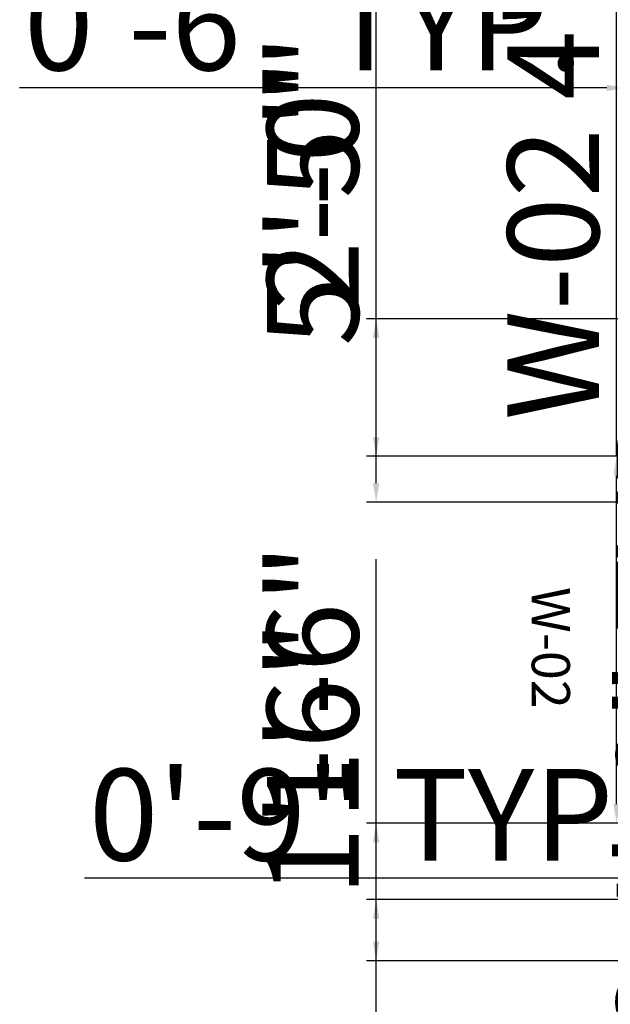
# Model space of a CAD drawing. Units: inches. Extents: x 2386 to 3029, y 792 to 1465.
# Tile 6 of 12: x 2386 to 2463, y 1140 to 1269. Entities that reach past the tile are written whole.
import ezdxf

# ---------------------------------------------------------------- set-up
doc = ezdxf.new("R2010")
doc.units = ezdxf.units.IN
doc.layers.add('A-DIMS', color=1, linetype='Continuous', lineweight=18)
doc.layers.add('A-TEXT', color=4, linetype='Continuous', lineweight=25)
doc.styles.get("Standard").update_dxf_attribs({"font": 'arial.ttf'})
doc.dimstyles.new('ISO-25', dxfattribs={"dimtxt": 12, "dimasz": 2.5, "dimexe": 1.25, "dimexo": 0.625, "dimtad": 1, "dimlunit": 4, "dimtxsty": 'Standard', "dimcen": 2.5, "dimadec": 0, "dimazin": 0, "dimtfac": 1, "dimtmove": 0, "dimatfit": 3, "dimfxl": 1, "dimarcsym": 0})

# ---------------------------------------------------------------- blocks, each defined once
blk = doc.blocks.new('*D38')
at = {"layer": 'A-DIMS', "color": 0, "lineweight": -2, "transparency": 16777216}
for p, q in [((2471.82, 1342.95), (2483.24, 1342.95)), ((2481.99, 1340.45), (2481.99, 1273.45)), ((2471.82, 1270.95), (2483.24, 1270.95)), ((2481.99, 1270.95), (2481.99, 1095.04))]:
    blk.add_line(p, q, dxfattribs=at)
at = {"layer": 'A-DIMS', "color": 0, "transparency": 16777216}
for points in [[(2481.57, 1340.45), (2482.41, 1340.45), (2481.99, 1342.95)], [(2481.57, 1273.45), (2482.41, 1273.45), (2481.99, 1270.95)]]:
    blk.add_solid(points, dxfattribs=at)
at = {"layer": 'Defpoints', "color": 0, "transparency": 16777216}
for p in [(2471.19, 1342.95), (2471.19, 1270.95), (2481.99, 1270.95)]:
    blk.add_point(p, dxfattribs=at)
at = {"layer": 'A-DIMS', "color": 0, "transparency": 16777216, "insert": (2475.16, 1181.74), "char_height": 12, "attachment_point": 5, "rotation": 90}
blk.add_mtext('HOOD W-01 6\'-0" TYP.', dxfattribs=at)
blk = doc.blocks.new('*D39')
at = {"layer": 'A-DIMS', "color": 0, "lineweight": -2, "transparency": 16777216}
for p, q in [((2465.19, 1270.32), (2465.19, 1258.9)), ((2471.19, 1270.32), (2471.19, 1258.9)), ((2462.69, 1260.15), (2385.79, 1260.15)), ((2471.19, 1260.15), (2465.19, 1260.15)), ((2473.69, 1260.15), (2476.19, 1260.15))]:
    blk.add_line(p, q, dxfattribs=at)
at = {"layer": 'A-DIMS', "color": 0, "transparency": 16777216}
for points in [[(2462.69, 1260.56), (2462.69, 1259.73), (2465.19, 1260.15)], [(2473.69, 1260.56), (2473.69, 1259.73), (2471.19, 1260.15)]]:
    blk.add_solid(points, dxfattribs=at)
at = {"layer": 'Defpoints', "color": 0, "transparency": 16777216}
for p in [(2465.19, 1270.95), (2471.19, 1270.95), (2465.19, 1260.15)]:
    blk.add_point(p, dxfattribs=at)
at = {"layer": 'A-DIMS', "color": 0, "transparency": 16777216, "insert": (2422.99, 1266.9), "char_height": 12, "attachment_point": 5}
blk.add_mtext('0\'-6" TYP.', dxfattribs=at)
blk = doc.blocks.new('*D40')
at = {"layer": 'A-DIMS', "color": 0, "lineweight": -2, "transparency": 16777216}
for p, q in [((2463.99, 1211.95), (2463.99, 1334.04)), ((2470.57, 1211.95), (2462.74, 1211.95)), ((2463.99, 1166.45), (2463.99, 1209.45)), ((2470.57, 1163.95), (2462.74, 1163.95))]:
    blk.add_line(p, q, dxfattribs=at)
at = {"layer": 'A-DIMS', "color": 0, "transparency": 16777216}
for points in [[(2463.57, 1209.45), (2464.41, 1209.45), (2463.99, 1211.95)], [(2463.57, 1166.45), (2464.41, 1166.45), (2463.99, 1163.95)]]:
    blk.add_solid(points, dxfattribs=at)
at = {"layer": 'Defpoints', "color": 0, "transparency": 16777216}
for p in [(2463.99, 1211.95), (2471.19, 1211.95), (2471.19, 1163.95)]:
    blk.add_point(p, dxfattribs=at)
at = {"layer": 'A-DIMS', "color": 0, "transparency": 16777216, "insert": (2457.24, 1274.25), "char_height": 12, "attachment_point": 5, "rotation": 90}
blk.add_mtext('W-02 4\'-0" TYP.', dxfattribs=at)
blk = doc.blocks.new('*D41')
at = {"layer": 'A-DIMS', "color": 0, "lineweight": -2, "transparency": 16777216}
for p, q in [((2471.19, 1163.32), (2471.19, 1155.5)), ((2480.19, 1163.32), (2480.19, 1155.5)), ((2471.19, 1156.75), (2394.29, 1156.75)), ((2477.69, 1156.75), (2473.69, 1156.75))]:
    blk.add_line(p, q, dxfattribs=at)
at = {"layer": 'A-DIMS', "color": 0, "transparency": 16777216}
for points in [[(2473.69, 1157.16), (2473.69, 1156.33), (2471.19, 1156.75)], [(2477.69, 1157.16), (2477.69, 1156.33), (2480.19, 1156.75)]]:
    blk.add_solid(points, dxfattribs=at)
at = {"layer": 'Defpoints', "color": 0, "transparency": 16777216}
for p in [(2471.19, 1163.95), (2480.19, 1163.95), (2471.19, 1156.75)]:
    blk.add_point(p, dxfattribs=at)
at = {"layer": 'A-DIMS', "color": 0, "transparency": 16777216, "insert": (2431.49, 1163.5), "char_height": 12, "attachment_point": 5}
blk.add_mtext('0\'-9" TYP.', dxfattribs=at)
blk = doc.blocks.new('*D44')
at = {"layer": 'A-DIMS', "color": 0, "lineweight": -2, "transparency": 16777216}
for p, q in [((2485.59, 1139.95), (2485.59, 1262.04)), ((2480.82, 1139.95), (2486.84, 1139.95)), ((2485.59, 1106.45), (2485.59, 1137.45)), ((2480.82, 1103.95), (2486.84, 1103.95))]:
    blk.add_line(p, q, dxfattribs=at)
at = {"layer": 'A-DIMS', "color": 0, "transparency": 16777216}
for points in [[(2485.17, 1137.45), (2486.01, 1137.45), (2485.59, 1139.95)], [(2485.17, 1106.45), (2486.01, 1106.45), (2485.59, 1103.95)]]:
    blk.add_solid(points, dxfattribs=at)
at = {"layer": 'Defpoints', "color": 0, "transparency": 16777216}
for p in [(2480.19, 1139.95), (2485.59, 1139.95), (2480.19, 1103.95)]:
    blk.add_point(p, dxfattribs=at)
at = {"layer": 'A-DIMS', "color": 0, "transparency": 16777216, "insert": (2478.83, 1202.25), "char_height": 12, "attachment_point": 5, "rotation": 90}
blk.add_mtext('W-03 3\'-0" TYP.', dxfattribs=at)
blk = doc.blocks.new('*D46')
at = {"layer": 'A-DIMS', "color": 0, "lineweight": -2, "transparency": 16777216}
for p, q in [((2478.39, 1049.95), (2478.39, 1225.86)), ((2471.82, 1049.95), (2479.64, 1049.95)), ((2478.39, 1004.45), (2478.39, 1047.45)), ((2471.82, 1001.95), (2479.64, 1001.95))]:
    blk.add_line(p, q, dxfattribs=at)
at = {"layer": 'A-DIMS', "color": 0, "transparency": 16777216}
for points in [[(2477.97, 1047.45), (2478.81, 1047.45), (2478.39, 1049.95)], [(2477.97, 1004.45), (2478.81, 1004.45), (2478.39, 1001.95)]]:
    blk.add_solid(points, dxfattribs=at)
at = {"layer": 'Defpoints', "color": 0, "transparency": 16777216}
for p in [(2471.19, 1049.95), (2478.39, 1049.95), (2471.19, 1001.95)]:
    blk.add_point(p, dxfattribs=at)
at = {"layer": 'A-DIMS', "color": 0, "transparency": 16777216, "insert": (2471.55, 1139.15), "char_height": 12, "attachment_point": 5, "rotation": 90}
blk.add_mtext('HOOD W-03 4\'-0" TYP.', dxfattribs=at)
blk = doc.blocks.new('*D64')
at = {"layer": 'A-DIMS', "color": 0, "lineweight": -2, "transparency": 16777216}
for p, q in [((2432.49, 1163.95), (2432.49, 1198.47)), ((2479.57, 1163.95), (2431.24, 1163.95)), ((2432.49, 1148.45), (2432.49, 1161.45)), ((2479.57, 1145.95), (2431.24, 1145.95))]:
    blk.add_line(p, q, dxfattribs=at)
at = {"layer": 'A-DIMS', "color": 0, "transparency": 16777216}
for points in [[(2432.07, 1161.45), (2432.91, 1161.45), (2432.49, 1163.95)], [(2432.07, 1148.45), (2432.91, 1148.45), (2432.49, 1145.95)]]:
    blk.add_solid(points, dxfattribs=at)
at = {"layer": 'Defpoints', "color": 0, "transparency": 16777216}
for p in [(2432.49, 1163.95), (2480.19, 1163.95), (2480.19, 1145.95)]:
    blk.add_point(p, dxfattribs=at)
at = {"layer": 'A-DIMS', "color": 0, "transparency": 16777216, "insert": (2425.74, 1182.46), "char_height": 12, "attachment_point": 5, "rotation": 90}
blk.add_mtext('1\'-6"', dxfattribs=at)
blk = doc.blocks.new('*D65')
at = {"layer": 'A-DIMS', "color": 0, "lineweight": -2, "transparency": 16777216}
for p, q in [((2470.57, 1276.95), (2431.24, 1276.95)), ((2432.49, 1214.45), (2432.49, 1274.45)), ((2470.57, 1211.95), (2431.24, 1211.95))]:
    blk.add_line(p, q, dxfattribs=at)
at = {"layer": 'A-DIMS', "color": 0, "transparency": 16777216}
for points in [[(2432.07, 1274.45), (2432.91, 1274.45), (2432.49, 1276.95)], [(2432.07, 1214.45), (2432.91, 1214.45), (2432.49, 1211.95)]]:
    blk.add_solid(points, dxfattribs=at)
at = {"layer": 'Defpoints', "color": 0, "transparency": 16777216}
for p in [(2432.49, 1276.95), (2471.19, 1276.95), (2471.19, 1211.95)]:
    blk.add_point(p, dxfattribs=at)
at = {"layer": 'A-DIMS', "color": 0, "transparency": 16777216, "insert": (2425.76, 1244.45), "char_height": 12, "attachment_point": 5, "rotation": 90}
blk.add_mtext('5\'-5"', dxfattribs=at)
blk = doc.blocks.new('*D81')
at = {"layer": 'A-DIMS', "color": 0, "lineweight": -2, "transparency": 16777216}
for p, q in [((2432.49, 1153.95), (2432.49, 1188.47)), ((2809.57, 1153.95), (2431.24, 1153.95)), ((2432.49, 1138.45), (2432.49, 1151.45)), ((2809.57, 1135.95), (2431.24, 1135.95))]:
    blk.add_line(p, q, dxfattribs=at)
at = {"layer": 'A-DIMS', "color": 0, "transparency": 16777216}
for points in [[(2432.07, 1151.45), (2432.91, 1151.45), (2432.49, 1153.95)], [(2432.07, 1138.45), (2432.91, 1138.45), (2432.49, 1135.95)]]:
    blk.add_solid(points, dxfattribs=at)
at = {"layer": 'Defpoints', "color": 0, "transparency": 16777216}
for p in [(2432.49, 1153.95), (2810.19, 1153.95), (2810.19, 1135.95)]:
    blk.add_point(p, dxfattribs=at)
at = {"layer": 'A-DIMS', "color": 0, "transparency": 16777216, "insert": (2425.74, 1172.46), "char_height": 12, "attachment_point": 5, "rotation": 90}
blk.add_mtext('1\'-6"', dxfattribs=at)
blk = doc.blocks.new('*D93')
at = {"layer": 'A-DIMS', "color": 0, "lineweight": -2, "transparency": 16777216}
for p, q in [((2432.49, 1229.95), (2432.49, 1265.8)), ((2587.57, 1229.95), (2431.24, 1229.95)), ((2432.49, 1208.45), (2432.49, 1227.45)), ((2587.57, 1205.95), (2431.24, 1205.95))]:
    blk.add_line(p, q, dxfattribs=at)
at = {"layer": 'A-DIMS', "color": 0, "transparency": 16777216}
for points in [[(2432.07, 1227.45), (2432.91, 1227.45), (2432.49, 1229.95)], [(2432.07, 1208.45), (2432.91, 1208.45), (2432.49, 1205.95)]]:
    blk.add_solid(points, dxfattribs=at)
at = {"layer": 'Defpoints', "color": 0, "transparency": 16777216}
for p in [(2432.49, 1229.95), (2588.19, 1229.95), (2588.19, 1205.95)]:
    blk.add_point(p, dxfattribs=at)
at = {"layer": 'A-DIMS', "color": 0, "transparency": 16777216, "insert": (2425.74, 1249.12), "char_height": 12, "attachment_point": 5, "rotation": 90}
blk.add_mtext('2\'-0"', dxfattribs=at)

msp = doc.modelspace()

# ---------------------------------------------------------------- texts
at = {"layer": 'A-TEXT', "insert": (2457.869, 1194.848), "char_height": 5, "attachment_point": 1, "rotation": 270}
msp.add_mtext_dynamic_manual_height_columns('W-02', width=38.22215, gutter_width=12.5, heights=[0], dxfattribs=at)

# ---------------------------------------------------------------- dimensions: what is measured, and where the dimension line sits
at = {"layer": 'A-DIMS'}
for base, p1, p2, angle, text, picture, middle in [((2481.99, 1270.948), (2471.19, 1342.948), (2471.19, 1270.948), 270, 'HOOD W-01 <> TYP.', '*D38', (2475.156, 1181.744)), ((2463.99, 1211.948), (2471.19, 1163.948), (2471.19, 1211.948), 90, 'W-02 <> TYP.', '*D40', (2457.238, 1274.246)), ((2465.19, 1260.148), (2471.19, 1270.948), (2465.19, 1270.948), 180, '<> TYP.', '*D39', (2422.992, 1266.9)), ((2485.59, 1139.948), (2480.19, 1103.948), (2480.19, 1139.948), 90, 'W-03 <> TYP.', '*D44', (2478.834, 1202.246)), ((2478.39, 1049.948), (2471.19, 1001.948), (2471.19, 1049.948), 90, 'HOOD W-03 <> TYP.', '*D46', (2471.552, 1139.152)), ((2471.19, 1156.748), (2480.19, 1163.948), (2471.19, 1163.948), 180, '<> TYP.', '*D41', (2431.492, 1163.5))]:
    dim = msp.add_linear_dim(base=base, p1=p1, p2=p2, angle=angle, text=text, dimstyle='ISO-25', override={"dimdec": 1, "dimlfac": 1, "dimrnd": 0, "dimzin": 1, "dimdsep": 46, "dimlunit": 4, "dimfrac": 2}, dxfattribs=at)
    dim.commit()
    dim.dimension.update_dxf_attribs({"geometry": picture, "text_midpoint": middle})
for base, p1, p2, picture, middle in [((2432.49, 1276.948), (2471.19, 1211.948), (2471.19, 1276.948), '*D65', (2425.763, 1244.448)), ((2432.49, 1229.948), (2588.19, 1205.948), (2588.19, 1229.948), '*D93', (2425.738, 1249.125)), ((2432.49, 1163.948), (2480.19, 1145.948), (2480.19, 1163.948), '*D64', (2425.738, 1182.458)), ((2432.49, 1153.948), (2810.19, 1135.948), (2810.19, 1153.948), '*D81', (2425.738, 1172.458))]:
    dim = msp.add_linear_dim(base=base, p1=p1, p2=p2, angle=90, dimstyle='ISO-25', override={"dimdec": 1, "dimlfac": 1, "dimrnd": 0, "dimzin": 1, "dimdsep": 46, "dimlunit": 4, "dimfrac": 2}, dxfattribs=at)
    dim.commit()
    dim.dimension.update_dxf_attribs({"geometry": picture, "text_midpoint": middle})

doc.saveas('drawing.dxf')
